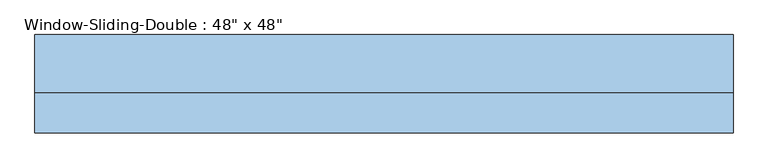
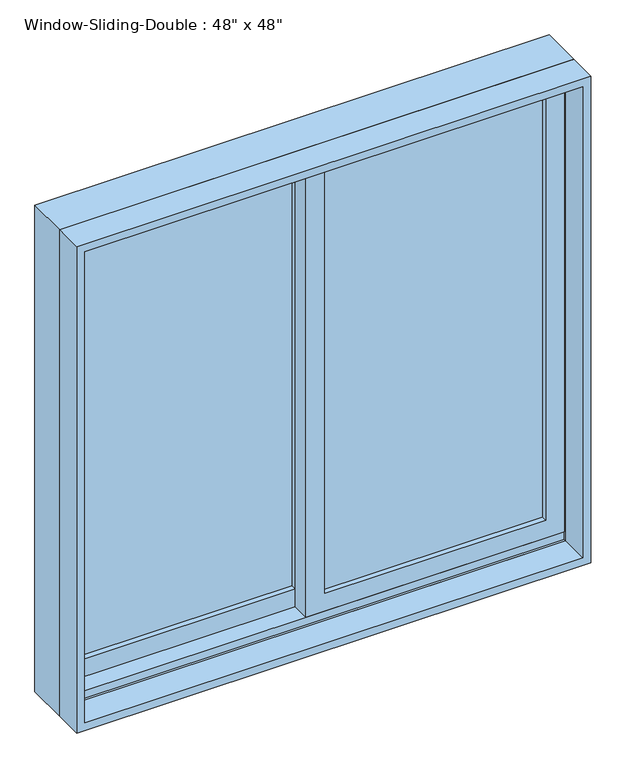
"""IFC4 building model written with IfcOpenShell, lengths in millimetres: window geometry."""

from ifc_helpers import new_model, si_unit, frame, origin, place, context, project, spatial, polyline, outline, extrude, faceted_brep, source, transform, mapped, element, save


def window_49fe3060(model_context):
    return source(origin(), model_context, "Body", "SolidModel", [
        extrude(outline(polyline([(952.5, 590.55), (2114.55, 590.55), (2114.55, -22.225), (952.5, -22.225), (952.5, 590.55)]), holes=[polyline([(996.95, 22.225), (2070.1, 22.225), (2070.1, 546.1), (996.95, 546.1), (996.95, 22.225)])]), frame((0.0, -3.81, 0.0), z_axis=(0.0, 1.0, 0.0), x_axis=(0.0, 0.0, 1.0)), (0.0, 0.0, 1.0), 44.45),
        extrude(outline(polyline([(933.45, -590.55), (933.45, 22.225), (2114.55, 22.225), (2114.55, -590.55), (933.45, -590.55)]), holes=[polyline([(2070.1, -22.225), (996.95, -22.225), (996.95, -546.1), (2070.1, -546.1), (2070.1, -22.225)])]), frame((0.0, 40.64, 0.0), z_axis=(0.0, 1.0, 0.0), x_axis=(0.0, 0.0, 1.0)), (0.0, 0.0, 1.0), 44.45),
        extrude(outline(polyline([(-22.225, 72.39), (-22.225, 66.04), (-546.1, 66.04), (-546.1, 72.39), (-22.225, 72.39)])), frame((0.0, 0.0, 996.95), z_axis=(0.0, 0.0, 1.0), x_axis=(1.0, 0.0, 0.0)), (0.0, 0.0, 1.0), 1073.15),
        extrude(outline(polyline([(-22.225, 59.69), (-22.225, 53.34), (-546.1, 53.34), (-546.1, 59.69), (-22.225, 59.69)])), frame((0.0, 0.0, 996.95), z_axis=(0.0, 0.0, 1.0), x_axis=(1.0, 0.0, 0.0)), (0.0, 0.0, 1.0), 1073.15),
        extrude(outline(polyline([(546.1, 27.94), (546.1, 21.59), (22.225, 21.59), (22.225, 27.94), (546.1, 27.94)])), frame((0.0, 0.0, 996.95), z_axis=(0.0, 0.0, 1.0), x_axis=(1.0, 0.0, 0.0)), (0.0, 0.0, 1.0), 1073.15),
        extrude(outline(polyline([(546.1, 15.24), (546.1, 8.89), (22.225, 8.89), (22.225, 15.24), (546.1, 15.24)])), frame((0.0, 0.0, 996.95), z_axis=(0.0, 0.0, 1.0), x_axis=(1.0, 0.0, 0.0)), (0.0, 0.0, 1.0), 1073.15),
        extrude(outline(polyline([(2133.6, -609.6), (914.4, -609.6), (914.4, 609.6), (2133.6, 609.6), (2133.6, -609.6)]), holes=[polyline([(2114.55, 590.55), (933.45, 590.55), (933.45, -590.55), (2114.55, -590.55), (2114.55, 590.55)])]), frame((0.0, -80.01, 0.0), z_axis=(0.0, 1.0, 0.0), x_axis=(0.0, 0.0, 1.0)), (0.0, 0.0, 1.0), 69.85),
        faceted_brep([(-609.6, -10.16, 914.4), (-609.6, 91.44, 914.4), (609.6, 91.44, 914.4), (609.6, -10.16, 914.4), (-568.6778905, 91.44, 2092.6778905), (-568.6778905, 85.09, 2092.6778905), (-568.6778905, 85.09, 933.45), (-568.6778905, 91.44, 933.45), (568.6778905, 85.09, 2092.6778905), (568.6778905, 85.09, 933.45), (590.55, 85.09, 933.45), (590.55, 85.09, 2114.55), (-590.55, 85.09, 2114.55), (-590.55, 85.09, 933.45), (-590.55, -10.16, 2114.55), (-590.55, -10.16, 933.45), (-590.55, -3.81, 933.45), (-590.55, -3.81, 952.5), (-590.55, 40.64, 952.5), (-590.55, 40.64, 933.45), (609.6, -10.16, 2133.6), (-609.6, -10.16, 2133.6), (590.55, -10.16, 2114.55), (590.55, -10.16, 933.45), (-609.6, 91.44, 2133.6), (609.6, 91.44, 2133.6), (568.6778905, 91.44, 933.45), (568.6778905, 91.44, 2092.6778905), (590.55, 40.64, 933.45), (590.55, 40.64, 952.5), (590.55, -3.81, 952.5), (590.55, -3.81, 933.45)], [[[0, 1, 2, 3]], [[4, 5, 6, 7]], [[5, 8, 9, 10, 11, 12, 13, 6]], [[12, 14, 15, 16, 17, 18, 19, 13]], [[0, 3, 20, 21], [22, 23, 15, 14]], [[24, 1, 0, 21]], [[2, 1, 24, 25], [4, 7, 26, 27]], [[5, 4, 27, 8]], [[12, 11, 22, 14]], [[21, 20, 25, 24]], [[8, 27, 26, 9]], [[22, 11, 10, 28, 29, 30, 31, 23]], [[20, 3, 2, 25]], [[26, 7, 6, 13, 19, 28, 10, 9]], [[28, 19, 18, 29]], [[29, 18, 17, 30]], [[30, 17, 16, 31]], [[15, 23, 31, 16]]]),
    ])


if __name__ == "__main__":
    model = new_model("IFC4")
    model_context = context("Model", 3, world=origin())
    ifc_project = project(units=[si_unit("LENGTHUNIT", "METRE", prefix="MILLI")], contexts=[model_context])
    site = spatial("IfcSite", under=ifc_project)
    building = spatial("IfcBuilding", under=site)
    placement = place(None, origin())
    window_shape = window_49fe3060(model_context)
    element("IfcWindow", 1, ObjectType="Window-Sliding-Double : 48\" x 48\"", at=placement, inside=building, context=model_context, shape_type="MappedRepresentation", body=[
        mapped(window_shape, transform((0.0, 0.0, 0.0), x_axis=(1.0, 0.0, 0.0), y_axis=(0.0, 1.0, 0.0), z_axis=(0.0, 0.0, 1.0))),
    ])
    save(model, "model.ifc")

# Revit data of these elements
# Type "Window-Sliding-Double : 48\" x 48\""
#   Type Mark = "23"
#   Fire Rating = "0.5h"
#   Assembly Code = "B2020100"
#   Analytic Construction = "Double glazing - domestic"
#   Window Inset [instance default] = 0' - 0"
#   Wall Thickness [instance default] = 0' - 6"
#   Visual Light Transmittance = 0.81
#   Thermal Resistance (R) = 1.8146 (h·ft²·°F)/BTU
#   Solar Heat Gain Coefficient = 0.76
#   Muntin Width = 1' - 8 5/8"
#   Muntin Height = 3' - 6 1/4"
#   Interior Wall Closure [instance default] = 0' - 2 3/4"
#   Heat Transfer Coefficient (U) = 0.5511 BTU/(h·ft²·°F)
#   Frame Extension [instance default] = 0' - 0 1/4"
#   Exterior Wall Closure [instance default] = 0' - 1 1/4"
#   Rough Width = 4' - 0 1/2"
#   Rough Height = 4' - 0 1/2"
#   Height = 4' - 0"
#   Extension Jamb [instance default] = 0' - 2 3/4"
#   Default Sill Height = 3' - 0"
#   Width = 4' - 0"
#   Interior Trim Visibility [instance default] = yes
#   Indicator Visibility [instance default] = yes
#   Exterior Trim Visibility [instance default] = yes
#   Muntin Visibility = yes
#   Extension Jamb Visibility [instance default] = yes
#   Muntin Pattern = Muntin Pattern_2x2 : Muntin Pattern_2x2
#   Interior Trim Material = Wood - Stained
#   Interior Trim = Trim-Window-Interior-Flat : Picture Frame
#   Interior Frame Material = Wood - Stained
#   Glass Panel Material = Glass
#   Exterior Trim Material = Clad - White
#   Exterior Trim = Trim-Window-Exterior-Flat : with Sill
#   Exterior Frame Material = Clad - White
#   Wall Closure = (empty or 0)
# Element 1 (IfcWindow, "Window-Sliding-Double : 48\" x 48\"")
#   Materials on its faces: "Wood - Stained", "Glass", "Clad - White"
# Materials
#   "Wood - Stained": class "Wood", colour RGB 224 178 126, transparency 0, Cost = 0
#   "Glass": class "Glass", colour RGB 0 128 192, transparency 0.75, Description = "Soda Lime Glass", Cost = 0
#   "Clad - White": class "Wood", colour RGB 242 242 238, transparency 0, Cost = 0
